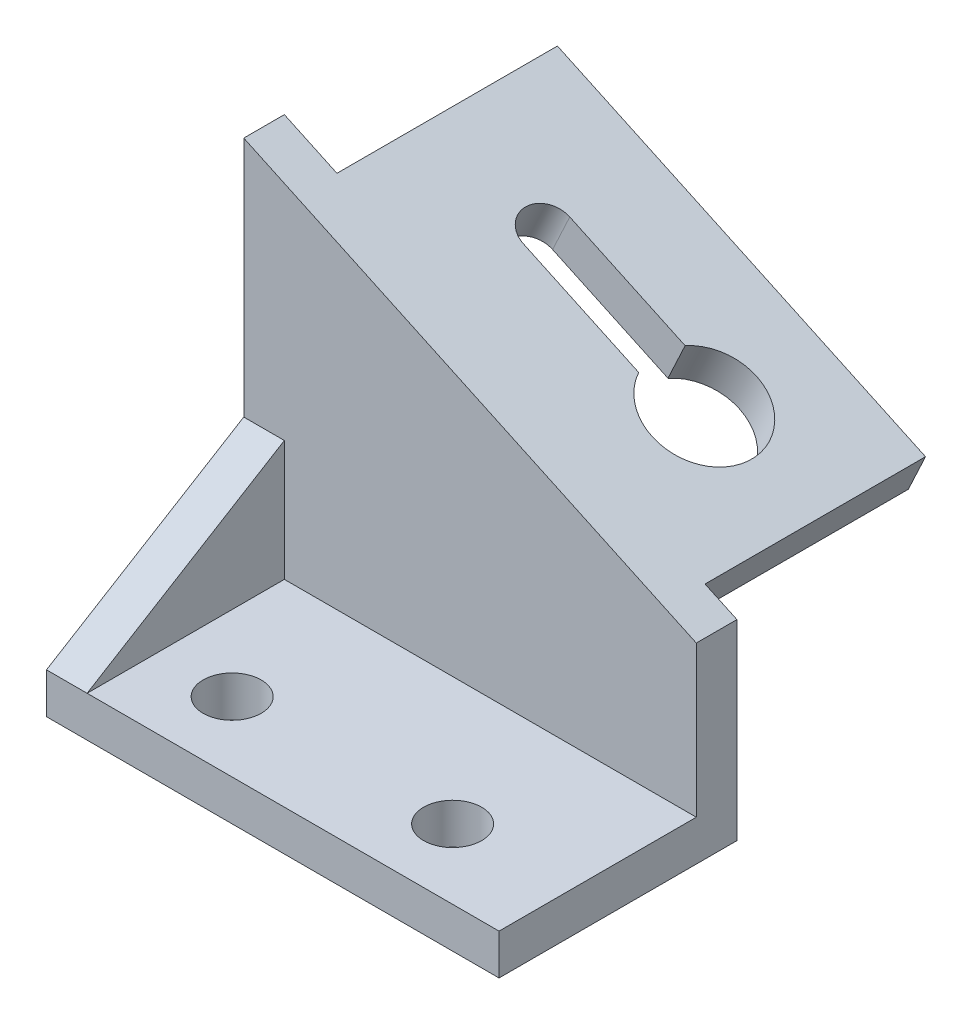
ISO-10303-21;
HEADER;
FILE_DESCRIPTION(('STEP AP214'),'2;1');
FILE_NAME('part.step','',(''),(''),'','','');
FILE_SCHEMA(('AUTOMOTIVE_DESIGN { 1 0 10303 214 1 1 1 1 }'));
ENDSEC;
DATA;
#1=APPLICATION_CONTEXT('core data for automotive mechanical design processes');
#2=APPLICATION_PROTOCOL_DEFINITION('international standard','automotive_design',2000,#1);
#3=PRODUCT_CONTEXT('',#1,'mechanical');
#4=PRODUCT('Part','Part','',(#3));
#5=PRODUCT_RELATED_PRODUCT_CATEGORY('part','',(#4));
#6=PRODUCT_DEFINITION_FORMATION('','',#4);
#7=PRODUCT_DEFINITION_CONTEXT('part definition',#1,'design');
#8=PRODUCT_DEFINITION('design','',#6,#7);
#9=PRODUCT_DEFINITION_SHAPE('','',#8);
#10=(LENGTH_UNIT() NAMED_UNIT(*) SI_UNIT(.MILLI.,.METRE.));
#11=(NAMED_UNIT(*) PLANE_ANGLE_UNIT() SI_UNIT($,.RADIAN.));
#12=(NAMED_UNIT(*) SI_UNIT($,.STERADIAN.) SOLID_ANGLE_UNIT());
#13=UNCERTAINTY_MEASURE_WITH_UNIT(LENGTH_MEASURE(1.E-05),#10,'distance_accuracy_value','');
#14=(GEOMETRIC_REPRESENTATION_CONTEXT(3) GLOBAL_UNCERTAINTY_ASSIGNED_CONTEXT((#13)) GLOBAL_UNIT_ASSIGNED_CONTEXT((#10,
#11,#12)) REPRESENTATION_CONTEXT('',''));
#15=CARTESIAN_POINT('',(0.,0.,0.));
#16=DIRECTION('',(0.,0.,1.));
#17=DIRECTION('',(1.,0.,0.));
#18=AXIS2_PLACEMENT_3D('',#15,#16,#17);
#19=CARTESIAN_POINT('',(-39.,7.,-20.5));
#20=DIRECTION('',(0.,0.,1.));
#21=DIRECTION('',(1.,0.,0.));
#22=AXIS2_PLACEMENT_3D('',#19,#20,#21);
#23=PLANE('',#22);
#24=DIRECTION('',(0.422618261740701,0.906307787036649,0.));
#25=VECTOR('',#24,1.);
#26=CARTESIAN_POINT('',(-32.8952499618184,58.8016602094265,-20.5));
#27=LINE('',#26,#25);
#28=CARTESIAN_POINT('',(-32.8952499618184,58.8016602094265,-20.5));
#29=VERTEX_POINT('',#28);
#30=CARTESIAN_POINT('',(-29.9369221296335,65.145814718683,-20.5));
#31=VERTEX_POINT('',#30);
#32=EDGE_CURVE('E202',#29,#31,#27,.T.);
#33=ORIENTED_EDGE('',*,*,#32,.F.);
#34=DIRECTION('',(0.906307787036649,-0.422618261740701,0.));
#35=VECTOR('',#34,1.);
#36=CARTESIAN_POINT('',(-32.8952499618184,58.8016602094265,-20.5));
#37=LINE('',#36,#35);
#38=CARTESIAN_POINT('',(30.5462951307471,29.2183818875774,-20.5));
#39=VERTEX_POINT('',#38);
#40=EDGE_CURVE('E193',#29,#39,#37,.T.);
#41=ORIENTED_EDGE('',*,*,#40,.T.);
#42=DIRECTION('',(0.422618261740701,0.906307787036649,0.));
#43=VECTOR('',#42,1.);
#44=CARTESIAN_POINT('',(30.5462951307471,29.2183818875774,-20.5));
#45=LINE('',#44,#43);
#46=CARTESIAN_POINT('',(33.504622962932,35.562536396834,-20.5));
#47=VERTEX_POINT('',#46);
#48=EDGE_CURVE('E216',#39,#47,#45,.T.);
#49=ORIENTED_EDGE('',*,*,#48,.T.);
#50=DIRECTION('',(0.906307787036649,-0.422618261740701,0.));
#51=VECTOR('',#50,1.);
#52=CARTESIAN_POINT('',(39.,33.,-20.5));
#53=LINE('',#52,#51);
#54=CARTESIAN_POINT('',(39.,33.,-20.5));
#55=VERTEX_POINT('',#54);
#56=EDGE_CURVE('E213',#47,#55,#53,.T.);
#57=ORIENTED_EDGE('',*,*,#56,.T.);
#58=DIRECTION('',(0.,-1.,0.));
#59=VECTOR('',#58,1.);
#60=CARTESIAN_POINT('',(39.,7.,-20.5));
#61=LINE('',#60,#59);
#62=CARTESIAN_POINT('',(39.,0.,-20.5));
#63=VERTEX_POINT('',#62);
#64=EDGE_CURVE('E50',#55,#63,#61,.T.);
#65=ORIENTED_EDGE('',*,*,#64,.T.);
#66=DIRECTION('',(-1.,0.,0.));
#67=VECTOR('',#66,1.);
#68=CARTESIAN_POINT('',(-39.,0.,-20.5));
#69=LINE('',#68,#67);
#70=CARTESIAN_POINT('',(-39.,0.,-20.5));
#71=VERTEX_POINT('',#70);
#72=EDGE_CURVE('E275',#63,#71,#69,.T.);
#73=ORIENTED_EDGE('',*,*,#72,.T.);
#74=DIRECTION('',(0.,-1.,0.));
#75=VECTOR('',#74,1.);
#76=CARTESIAN_POINT('',(-39.,7.,-20.5));
#77=LINE('',#76,#75);
#78=CARTESIAN_POINT('',(-39.,69.37199733609,-20.5));
#79=VERTEX_POINT('',#78);
#80=EDGE_CURVE('E282',#79,#71,#77,.T.);
#81=ORIENTED_EDGE('',*,*,#80,.F.);
#82=EDGE_CURVE('E224',#79,#31,#53,.T.);
#83=ORIENTED_EDGE('',*,*,#82,.T.);
#84=EDGE_LOOP('',(#33,#41,#49,#57,#65,#73,#81,#83));
#85=FACE_BOUND('',#84,.T.);
#86=ADVANCED_FACE('F39',(#85),#23,.F.);
#87=CARTESIAN_POINT('',(0.,7.,0.));
#88=DIRECTION('',(0.,1.,0.));
#89=DIRECTION('',(0.,0.,1.));
#90=AXIS2_PLACEMENT_3D('',#87,#88,#89);
#91=PLANE('',#90);
#92=CARTESIAN_POINT('',(-19.,7.,8.5));
#93=DIRECTION('',(0.,1.,0.));
#94=DIRECTION('',(0.,0.,1.));
#95=AXIS2_PLACEMENT_3D('',#92,#93,#94);
#96=CIRCLE('',#95,5.);
#97=CARTESIAN_POINT('',(-19.,7.,13.5));
#98=VERTEX_POINT('',#97);
#99=EDGE_CURVE('E254',#98,#98,#96,.T.);
#100=ORIENTED_EDGE('',*,*,#99,.F.);
#101=EDGE_LOOP('',(#100));
#102=FACE_BOUND('',#101,.T.);
#103=CARTESIAN_POINT('',(19.,7.,8.5));
#104=DIRECTION('',(0.,1.,0.));
#105=DIRECTION('',(0.,0.,1.));
#106=AXIS2_PLACEMENT_3D('',#103,#104,#105);
#107=CIRCLE('',#106,5.);
#108=CARTESIAN_POINT('',(19.,7.,13.5));
#109=VERTEX_POINT('',#108);
#110=EDGE_CURVE('E246',#109,#109,#107,.T.);
#111=ORIENTED_EDGE('',*,*,#110,.F.);
#112=EDGE_LOOP('',(#111));
#113=FACE_BOUND('',#112,.T.);
#114=DIRECTION('',(0.,0.,-1.));
#115=VECTOR('',#114,1.);
#116=CARTESIAN_POINT('',(39.,7.,-20.5));
#117=LINE('',#116,#115);
#118=CARTESIAN_POINT('',(39.,7.,20.5));
#119=VERTEX_POINT('',#118);
#120=CARTESIAN_POINT('',(39.,7.,-13.5));
#121=VERTEX_POINT('',#120);
#122=EDGE_CURVE('E261',#119,#121,#117,.T.);
#123=ORIENTED_EDGE('',*,*,#122,.T.);
#124=DIRECTION('',(-1.,0.,0.));
#125=VECTOR('',#124,1.);
#126=CARTESIAN_POINT('',(-39.,7.,-13.5));
#127=LINE('',#126,#125);
#128=CARTESIAN_POINT('',(-32.,7.,-13.5));
#129=VERTEX_POINT('',#128);
#130=EDGE_CURVE('E218',#121,#129,#127,.T.);
#131=ORIENTED_EDGE('',*,*,#130,.T.);
#132=DIRECTION('',(0.,0.,1.));
#133=VECTOR('',#132,1.);
#134=CARTESIAN_POINT('',(-32.,7.,-20.5));
#135=LINE('',#134,#133);
#136=CARTESIAN_POINT('',(-32.,7.,20.5));
#137=VERTEX_POINT('',#136);
#138=EDGE_CURVE('E243',#129,#137,#135,.T.);
#139=ORIENTED_EDGE('',*,*,#138,.T.);
#140=DIRECTION('',(1.,0.,0.));
#141=VECTOR('',#140,1.);
#142=CARTESIAN_POINT('',(-39.,7.,20.5));
#143=LINE('',#142,#141);
#144=EDGE_CURVE('E262',#137,#119,#143,.T.);
#145=ORIENTED_EDGE('',*,*,#144,.T.);
#146=EDGE_LOOP('',(#123,#131,#139,#145));
#147=FACE_BOUND('',#146,.T.);
#148=ADVANCED_FACE('F320',(#102,#113,#147),#91,.T.);
#149=CARTESIAN_POINT('',(0.,0.,0.));
#150=DIRECTION('',(0.,1.,0.));
#151=DIRECTION('',(0.,0.,1.));
#152=AXIS2_PLACEMENT_3D('',#149,#150,#151);
#153=PLANE('',#152);
#154=DIRECTION('',(0.,0.,-1.));
#155=VECTOR('',#154,1.);
#156=CARTESIAN_POINT('',(39.,0.,-20.5));
#157=LINE('',#156,#155);
#158=CARTESIAN_POINT('',(39.,0.,20.5));
#159=VERTEX_POINT('',#158);
#160=EDGE_CURVE('E256',#159,#63,#157,.T.);
#161=ORIENTED_EDGE('',*,*,#160,.F.);
#162=DIRECTION('',(1.,0.,0.));
#163=VECTOR('',#162,1.);
#164=CARTESIAN_POINT('',(-39.,0.,20.5));
#165=LINE('',#164,#163);
#166=CARTESIAN_POINT('',(-39.,0.,20.5));
#167=VERTEX_POINT('',#166);
#168=EDGE_CURVE('E264',#167,#159,#165,.T.);
#169=ORIENTED_EDGE('',*,*,#168,.F.);
#170=DIRECTION('',(0.,0.,1.));
#171=VECTOR('',#170,1.);
#172=CARTESIAN_POINT('',(-39.,0.,-20.5));
#173=LINE('',#172,#171);
#174=EDGE_CURVE('E274',#71,#167,#173,.T.);
#175=ORIENTED_EDGE('',*,*,#174,.F.);
#176=ORIENTED_EDGE('',*,*,#72,.F.);
#177=EDGE_LOOP('',(#161,#169,#175,#176));
#178=FACE_BOUND('',#177,.T.);
#179=CARTESIAN_POINT('',(-19.,0.,8.5));
#180=DIRECTION('',(0.,1.,0.));
#181=DIRECTION('',(0.,0.,1.));
#182=AXIS2_PLACEMENT_3D('',#179,#180,#181);
#183=CIRCLE('',#182,5.);
#184=CARTESIAN_POINT('',(-19.,0.,13.5));
#185=VERTEX_POINT('',#184);
#186=EDGE_CURVE('E252',#185,#185,#183,.T.);
#187=ORIENTED_EDGE('',*,*,#186,.T.);
#188=EDGE_LOOP('',(#187));
#189=FACE_BOUND('',#188,.T.);
#190=CARTESIAN_POINT('',(19.,0.,8.5));
#191=DIRECTION('',(0.,1.,0.));
#192=DIRECTION('',(0.,0.,1.));
#193=AXIS2_PLACEMENT_3D('',#190,#191,#192);
#194=CIRCLE('',#193,5.);
#195=CARTESIAN_POINT('',(19.,0.,13.5));
#196=VERTEX_POINT('',#195);
#197=EDGE_CURVE('E247',#196,#196,#194,.T.);
#198=ORIENTED_EDGE('',*,*,#197,.T.);
#199=EDGE_LOOP('',(#198));
#200=FACE_BOUND('',#199,.T.);
#201=ADVANCED_FACE('F298',(#178,#189,#200),#153,.F.);
#202=CARTESIAN_POINT('',(39.,7.,-20.5));
#203=DIRECTION('',(-1.,0.,0.));
#204=DIRECTION('',(0.,0.,1.));
#205=AXIS2_PLACEMENT_3D('',#202,#203,#204);
#206=PLANE('',#205);
#207=ORIENTED_EDGE('',*,*,#160,.T.);
#208=ORIENTED_EDGE('',*,*,#64,.F.);
#209=DIRECTION('',(0.,0.,-1.));
#210=VECTOR('',#209,1.);
#211=CARTESIAN_POINT('',(39.,33.,-13.5));
#212=LINE('',#211,#210);
#213=CARTESIAN_POINT('',(39.,33.,-13.5));
#214=VERTEX_POINT('',#213);
#215=EDGE_CURVE('E231',#214,#55,#212,.T.);
#216=ORIENTED_EDGE('',*,*,#215,.F.);
#217=DIRECTION('',(0.,-1.,0.));
#218=VECTOR('',#217,1.);
#219=CARTESIAN_POINT('',(39.,7.,-13.5));
#220=LINE('',#219,#218);
#221=EDGE_CURVE('E227',#214,#121,#220,.T.);
#222=ORIENTED_EDGE('',*,*,#221,.T.);
#223=ORIENTED_EDGE('',*,*,#122,.F.);
#224=DIRECTION('',(0.,-1.,0.));
#225=VECTOR('',#224,1.);
#226=CARTESIAN_POINT('',(39.,7.,20.5));
#227=LINE('',#226,#225);
#228=EDGE_CURVE('E267',#119,#159,#227,.T.);
#229=ORIENTED_EDGE('',*,*,#228,.T.);
#230=EDGE_LOOP('',(#207,#208,#216,#222,#223,#229));
#231=FACE_BOUND('',#230,.T.);
#232=ADVANCED_FACE('F41',(#231),#206,.F.);
#233=CARTESIAN_POINT('',(-39.,7.,-20.5));
#234=DIRECTION('',(1.,0.,0.));
#235=DIRECTION('',(0.,0.,-1.));
#236=AXIS2_PLACEMENT_3D('',#233,#234,#235);
#237=PLANE('',#236);
#238=ORIENTED_EDGE('',*,*,#80,.T.);
#239=ORIENTED_EDGE('',*,*,#174,.T.);
#240=DIRECTION('',(0.,-1.,0.));
#241=VECTOR('',#240,1.);
#242=CARTESIAN_POINT('',(-39.,7.,20.5));
#243=LINE('',#242,#241);
#244=CARTESIAN_POINT('',(-39.,7.,20.5));
#245=VERTEX_POINT('',#244);
#246=EDGE_CURVE('E278',#245,#167,#243,.T.);
#247=ORIENTED_EDGE('',*,*,#246,.F.);
#248=DIRECTION('',(0.,0.520607424264656,-0.853796175794036));
#249=VECTOR('',#248,1.);
#250=CARTESIAN_POINT('',(-39.,7.,20.5));
#251=LINE('',#250,#249);
#252=CARTESIAN_POINT('',(-39.,27.7317073170732,-13.5));
#253=VERTEX_POINT('',#252);
#254=EDGE_CURVE('E238',#245,#253,#251,.T.);
#255=ORIENTED_EDGE('',*,*,#254,.T.);
#256=DIRECTION('',(0.,1.,0.));
#257=VECTOR('',#256,1.);
#258=CARTESIAN_POINT('',(-39.,69.37199733609,-13.5));
#259=LINE('',#258,#257);
#260=CARTESIAN_POINT('',(-39.,69.37199733609,-13.5));
#261=VERTEX_POINT('',#260);
#262=EDGE_CURVE('E225',#253,#261,#259,.T.);
#263=ORIENTED_EDGE('',*,*,#262,.T.);
#264=DIRECTION('',(0.,0.,-1.));
#265=VECTOR('',#264,1.);
#266=CARTESIAN_POINT('',(-39.,69.37199733609,-13.5));
#267=LINE('',#266,#265);
#268=EDGE_CURVE('E232',#261,#79,#267,.T.);
#269=ORIENTED_EDGE('',*,*,#268,.T.);
#270=EDGE_LOOP('',(#238,#239,#247,#255,#263,#269));
#271=FACE_BOUND('',#270,.T.);
#272=ADVANCED_FACE('F296',(#271),#237,.F.);
#273=CARTESIAN_POINT('',(-39.,7.,20.5));
#274=DIRECTION('',(0.,0.,-1.));
#275=DIRECTION('',(-1.,0.,0.));
#276=AXIS2_PLACEMENT_3D('',#273,#274,#275);
#277=PLANE('',#276);
#278=ORIENTED_EDGE('',*,*,#168,.T.);
#279=ORIENTED_EDGE('',*,*,#228,.F.);
#280=ORIENTED_EDGE('',*,*,#144,.F.);
#281=EDGE_CURVE('E266',#245,#137,#143,.T.);
#282=ORIENTED_EDGE('',*,*,#281,.F.);
#283=ORIENTED_EDGE('',*,*,#246,.T.);
#284=EDGE_LOOP('',(#278,#279,#280,#282,#283));
#285=FACE_BOUND('',#284,.T.);
#286=ADVANCED_FACE('F305',(#285),#277,.F.);
#287=CARTESIAN_POINT('',(-19.,7.,8.5));
#288=DIRECTION('',(0.,-1.,0.));
#289=DIRECTION('',(0.,0.,-1.));
#290=AXIS2_PLACEMENT_3D('',#287,#288,#289);
#291=CYLINDRICAL_SURFACE('',#290,5.);
#292=ORIENTED_EDGE('',*,*,#99,.T.);
#293=EDGE_LOOP('',(#292));
#294=FACE_BOUND('',#293,.T.);
#295=ORIENTED_EDGE('',*,*,#186,.F.);
#296=EDGE_LOOP('',(#295));
#297=FACE_BOUND('',#296,.T.);
#298=ADVANCED_FACE('F344',(#294,#297),#291,.F.);
#299=CARTESIAN_POINT('',(19.,7.,8.5));
#300=DIRECTION('',(0.,-1.,0.));
#301=DIRECTION('',(0.,0.,-1.));
#302=AXIS2_PLACEMENT_3D('',#299,#300,#301);
#303=CYLINDRICAL_SURFACE('',#302,5.);
#304=ORIENTED_EDGE('',*,*,#110,.T.);
#305=EDGE_LOOP('',(#304));
#306=FACE_BOUND('',#305,.T.);
#307=ORIENTED_EDGE('',*,*,#197,.F.);
#308=EDGE_LOOP('',(#307));
#309=FACE_BOUND('',#308,.T.);
#310=ADVANCED_FACE('F328',(#306,#309),#303,.F.);
#311=CARTESIAN_POINT('',(-32.,7.,20.5));
#312=DIRECTION('',(0.,0.853796175794036,0.520607424264656));
#313=DIRECTION('',(0.,-0.520607424264656,0.853796175794036));
#314=AXIS2_PLACEMENT_3D('',#311,#312,#313);
#315=PLANE('',#314);
#316=DIRECTION('',(1.,0.,0.));
#317=VECTOR('',#316,1.);
#318=CARTESIAN_POINT('',(-32.,27.7317073170732,-13.5));
#319=LINE('',#318,#317);
#320=CARTESIAN_POINT('',(-32.,27.7317073170732,-13.5));
#321=VERTEX_POINT('',#320);
#322=EDGE_CURVE('E64',#253,#321,#319,.T.);
#323=ORIENTED_EDGE('',*,*,#322,.F.);
#324=ORIENTED_EDGE('',*,*,#254,.F.);
#325=ORIENTED_EDGE('',*,*,#281,.T.);
#326=DIRECTION('',(0.,0.520607424264656,-0.853796175794036));
#327=VECTOR('',#326,1.);
#328=CARTESIAN_POINT('',(-32.,7.,20.5));
#329=LINE('',#328,#327);
#330=EDGE_CURVE('E242',#137,#321,#329,.T.);
#331=ORIENTED_EDGE('',*,*,#330,.T.);
#332=EDGE_LOOP('',(#323,#324,#325,#331));
#333=FACE_BOUND('',#332,.T.);
#334=ADVANCED_FACE('F308',(#333),#315,.T.);
#335=CARTESIAN_POINT('',(-32.,0.,0.));
#336=DIRECTION('',(-1.,0.,0.));
#337=DIRECTION('',(0.,0.,1.));
#338=AXIS2_PLACEMENT_3D('',#335,#336,#337);
#339=PLANE('',#338);
#340=ORIENTED_EDGE('',*,*,#138,.F.);
#341=DIRECTION('',(0.,1.,0.));
#342=VECTOR('',#341,1.);
#343=CARTESIAN_POINT('',(-32.,0.,-13.5));
#344=LINE('',#343,#342);
#345=EDGE_CURVE('E11',#129,#321,#344,.T.);
#346=ORIENTED_EDGE('',*,*,#345,.T.);
#347=ORIENTED_EDGE('',*,*,#330,.F.);
#348=EDGE_LOOP('',(#340,#346,#347));
#349=FACE_BOUND('',#348,.T.);
#350=ADVANCED_FACE('F319',(#349),#339,.F.);
#351=CARTESIAN_POINT('',(39.,33.,-13.5));
#352=DIRECTION('',(0.422618261740701,0.906307787036649,0.));
#353=DIRECTION('',(-0.906307787036649,0.422618261740701,0.));
#354=AXIS2_PLACEMENT_3D('',#351,#352,#353);
#355=PLANE('',#354);
#356=ORIENTED_EDGE('',*,*,#82,.F.);
#357=ORIENTED_EDGE('',*,*,#268,.F.);
#358=DIRECTION('',(0.906307787036649,-0.422618261740701,0.));
#359=VECTOR('',#358,1.);
#360=CARTESIAN_POINT('',(39.,33.,-13.5));
#361=LINE('',#360,#359);
#362=EDGE_CURVE('E223',#261,#214,#361,.T.);
#363=ORIENTED_EDGE('',*,*,#362,.T.);
#364=ORIENTED_EDGE('',*,*,#215,.T.);
#365=ORIENTED_EDGE('',*,*,#56,.F.);
#366=DIRECTION('',(0.,0.,-1.));
#367=VECTOR('',#366,1.);
#368=CARTESIAN_POINT('',(33.504622962932,35.562536396834,-20.5));
#369=LINE('',#368,#367);
#370=CARTESIAN_POINT('',(33.504622962932,35.562536396834,-58.5));
#371=VERTEX_POINT('',#370);
#372=EDGE_CURVE('E53',#47,#371,#369,.T.);
#373=ORIENTED_EDGE('',*,*,#372,.T.);
#374=DIRECTION('',(-0.906307787036649,0.422618261740701,0.));
#375=VECTOR('',#374,1.);
#376=CARTESIAN_POINT('',(-29.9369221296335,65.145814718683,-58.5));
#377=LINE('',#376,#375);
#378=CARTESIAN_POINT('',(-29.9369221296335,65.145814718683,-58.5));
#379=VERTEX_POINT('',#378);
#380=EDGE_CURVE('E198',#371,#379,#377,.T.);
#381=ORIENTED_EDGE('',*,*,#380,.T.);
#382=DIRECTION('',(0.,0.,1.));
#383=VECTOR('',#382,1.);
#384=CARTESIAN_POINT('',(-29.9369221296335,65.145814718683,-20.5));
#385=LINE('',#384,#383);
#386=EDGE_CURVE('E187',#379,#31,#385,.T.);
#387=ORIENTED_EDGE('',*,*,#386,.T.);
#388=EDGE_LOOP('',(#356,#357,#363,#364,#365,#373,#381,#387));
#389=FACE_BOUND('',#388,.T.);
#390=DIRECTION('',(0.906307787036649,-0.422618261740701,0.));
#391=VECTOR('',#390,1.);
#392=CARTESIAN_POINT('',(-11.8107663889005,56.693449483869,-34.5));
#393=LINE('',#392,#391);
#394=CARTESIAN_POINT('',(-11.8107663889005,56.693449483869,-34.5));
#395=VERTEX_POINT('',#394);
#396=CARTESIAN_POINT('',(8.07158024381943,47.4221589869394,-34.5));
#397=VERTEX_POINT('',#396);
#398=EDGE_CURVE('E185',#395,#397,#393,.T.);
#399=ORIENTED_EDGE('',*,*,#398,.F.);
#400=CARTESIAN_POINT('',(-11.8107663889005,56.693449483869,-38.5));
#401=DIRECTION('',(0.422618261740701,0.906307787036649,0.));
#402=DIRECTION('',(-0.906307787036649,0.422618261740701,0.));
#403=AXIS2_PLACEMENT_3D('',#400,#401,#402);
#404=CIRCLE('',#403,4.);
#405=CARTESIAN_POINT('',(-11.8107663889005,56.693449483869,-42.5));
#406=VERTEX_POINT('',#405);
#407=EDGE_CURVE('E154',#406,#395,#404,.T.);
#408=ORIENTED_EDGE('',*,*,#407,.F.);
#409=DIRECTION('',(-0.906307787036649,0.422618261740701,0.));
#410=VECTOR('',#409,1.);
#411=CARTESIAN_POINT('',(-11.8107663889005,56.693449483869,-42.5));
#412=LINE('',#411,#410);
#413=CARTESIAN_POINT('',(8.07158024381943,47.4221589869394,-42.5));
#414=VERTEX_POINT('',#413);
#415=EDGE_CURVE('E172',#414,#406,#412,.T.);
#416=ORIENTED_EDGE('',*,*,#415,.F.);
#417=CARTESIAN_POINT('',(15.378467222199,44.014901631648,-38.5));
#418=DIRECTION('',(0.422618261740701,0.906307787036649,0.));
#419=DIRECTION('',(-0.906307787036649,0.422618261740701,0.));
#420=AXIS2_PLACEMENT_3D('',#417,#418,#419);
#421=CIRCLE('',#420,9.);
#422=EDGE_CURVE('E177',#397,#414,#421,.T.);
#423=ORIENTED_EDGE('',*,*,#422,.F.);
#424=EDGE_LOOP('',(#399,#408,#416,#423));
#425=FACE_BOUND('',#424,.T.);
#426=ADVANCED_FACE('F315',(#389,#425),#355,.T.);
#427=CARTESIAN_POINT('',(0.,0.,-13.5));
#428=DIRECTION('',(0.,0.,1.));
#429=DIRECTION('',(1.,0.,0.));
#430=AXIS2_PLACEMENT_3D('',#427,#428,#429);
#431=PLANE('',#430);
#432=ORIENTED_EDGE('',*,*,#262,.F.);
#433=ORIENTED_EDGE('',*,*,#322,.T.);
#434=ORIENTED_EDGE('',*,*,#345,.F.);
#435=ORIENTED_EDGE('',*,*,#130,.F.);
#436=ORIENTED_EDGE('',*,*,#221,.F.);
#437=ORIENTED_EDGE('',*,*,#362,.F.);
#438=EDGE_LOOP('',(#432,#433,#434,#435,#436,#437));
#439=FACE_BOUND('',#438,.T.);
#440=ADVANCED_FACE('F312',(#439),#431,.T.);
#441=CARTESIAN_POINT('',(-32.8952499618184,58.8016602094265,-20.5));
#442=DIRECTION('',(-0.906307787036649,0.422618261740701,0.));
#443=DIRECTION('',(-0.422618261740701,-0.906307787036649,0.));
#444=AXIS2_PLACEMENT_3D('',#441,#442,#443);
#445=PLANE('',#444);
#446=ORIENTED_EDGE('',*,*,#386,.F.);
#447=DIRECTION('',(0.422618261740701,0.906307787036649,0.));
#448=VECTOR('',#447,1.);
#449=CARTESIAN_POINT('',(-32.8952499618184,58.8016602094265,-58.5));
#450=LINE('',#449,#448);
#451=CARTESIAN_POINT('',(-32.8952499618184,58.8016602094265,-58.5));
#452=VERTEX_POINT('',#451);
#453=EDGE_CURVE('E211',#452,#379,#450,.T.);
#454=ORIENTED_EDGE('',*,*,#453,.F.);
#455=DIRECTION('',(0.,0.,1.));
#456=VECTOR('',#455,1.);
#457=CARTESIAN_POINT('',(-32.8952499618184,58.8016602094265,-20.5));
#458=LINE('',#457,#456);
#459=EDGE_CURVE('E194',#452,#29,#458,.T.);
#460=ORIENTED_EDGE('',*,*,#459,.T.);
#461=ORIENTED_EDGE('',*,*,#32,.T.);
#462=EDGE_LOOP('',(#446,#454,#460,#461));
#463=FACE_BOUND('',#462,.T.);
#464=ADVANCED_FACE('F408',(#463),#445,.T.);
#465=CARTESIAN_POINT('',(-32.8952499618184,58.8016602094265,-58.5));
#466=DIRECTION('',(0.,0.,-1.));
#467=DIRECTION('',(-1.,0.,0.));
#468=AXIS2_PLACEMENT_3D('',#465,#466,#467);
#469=PLANE('',#468);
#470=ORIENTED_EDGE('',*,*,#380,.F.);
#471=DIRECTION('',(0.422618261740701,0.906307787036649,0.));
#472=VECTOR('',#471,1.);
#473=CARTESIAN_POINT('',(30.5462951307471,29.2183818875774,-58.5));
#474=LINE('',#473,#472);
#475=CARTESIAN_POINT('',(30.5462951307471,29.2183818875774,-58.5));
#476=VERTEX_POINT('',#475);
#477=EDGE_CURVE('E212',#476,#371,#474,.T.);
#478=ORIENTED_EDGE('',*,*,#477,.F.);
#479=DIRECTION('',(-0.906307787036649,0.422618261740701,0.));
#480=VECTOR('',#479,1.);
#481=CARTESIAN_POINT('',(-32.8952499618184,58.8016602094265,-58.5));
#482=LINE('',#481,#480);
#483=EDGE_CURVE('E205',#476,#452,#482,.T.);
#484=ORIENTED_EDGE('',*,*,#483,.T.);
#485=ORIENTED_EDGE('',*,*,#453,.T.);
#486=EDGE_LOOP('',(#470,#478,#484,#485));
#487=FACE_BOUND('',#486,.T.);
#488=ADVANCED_FACE('F423',(#487),#469,.T.);
#489=CARTESIAN_POINT('',(30.5462951307471,29.2183818875774,-20.5));
#490=DIRECTION('',(0.906307787036649,-0.422618261740701,0.));
#491=DIRECTION('',(0.422618261740701,0.906307787036649,0.));
#492=AXIS2_PLACEMENT_3D('',#489,#490,#491);
#493=PLANE('',#492);
#494=ORIENTED_EDGE('',*,*,#372,.F.);
#495=ORIENTED_EDGE('',*,*,#48,.F.);
#496=DIRECTION('',(0.,0.,-1.));
#497=VECTOR('',#496,1.);
#498=CARTESIAN_POINT('',(30.5462951307471,29.2183818875774,-20.5));
#499=LINE('',#498,#497);
#500=EDGE_CURVE('E200',#39,#476,#499,.T.);
#501=ORIENTED_EDGE('',*,*,#500,.T.);
#502=ORIENTED_EDGE('',*,*,#477,.T.);
#503=EDGE_LOOP('',(#494,#495,#501,#502));
#504=FACE_BOUND('',#503,.T.);
#505=ADVANCED_FACE('F429',(#504),#493,.T.);
#506=CARTESIAN_POINT('',(16.6470470903908,35.6997076913915,0.));
#507=DIRECTION('',(-0.422618261740701,-0.906307787036649,0.));
#508=DIRECTION('',(0.906307787036649,-0.422618261740701,0.));
#509=AXIS2_PLACEMENT_3D('',#506,#507,#508);
#510=PLANE('',#509);
#511=CARTESIAN_POINT('',(-14.7690942210854,50.3492949746125,-38.5));
#512=DIRECTION('',(0.422618261740701,0.906307787036649,0.));
#513=DIRECTION('',(-0.906307787036649,0.422618261740701,0.));
#514=AXIS2_PLACEMENT_3D('',#511,#512,#513);
#515=CIRCLE('',#514,4.);
#516=CARTESIAN_POINT('',(-14.7690942210854,50.3492949746125,-42.5));
#517=VERTEX_POINT('',#516);
#518=CARTESIAN_POINT('',(-14.7690942210854,50.3492949746125,-34.5));
#519=VERTEX_POINT('',#518);
#520=EDGE_CURVE('E155',#517,#519,#515,.T.);
#521=ORIENTED_EDGE('',*,*,#520,.T.);
#522=DIRECTION('',(0.906307787036649,-0.422618261740701,0.));
#523=VECTOR('',#522,1.);
#524=CARTESIAN_POINT('',(-14.7690942210854,50.3492949746125,-34.5));
#525=LINE('',#524,#523);
#526=CARTESIAN_POINT('',(5.11325241163458,41.0780044776829,-34.5));
#527=VERTEX_POINT('',#526);
#528=EDGE_CURVE('E163',#519,#527,#525,.T.);
#529=ORIENTED_EDGE('',*,*,#528,.T.);
#530=CARTESIAN_POINT('',(12.4201393900141,37.6707471223914,-38.5));
#531=DIRECTION('',(0.422618261740701,0.906307787036649,0.));
#532=DIRECTION('',(-0.906307787036649,0.422618261740701,0.));
#533=AXIS2_PLACEMENT_3D('',#530,#531,#532);
#534=CIRCLE('',#533,9.);
#535=CARTESIAN_POINT('',(5.11325241163452,41.0780044776829,-42.5));
#536=VERTEX_POINT('',#535);
#537=EDGE_CURVE('E169',#527,#536,#534,.T.);
#538=ORIENTED_EDGE('',*,*,#537,.T.);
#539=DIRECTION('',(-0.906307787036649,0.422618261740701,0.));
#540=VECTOR('',#539,1.);
#541=CARTESIAN_POINT('',(-14.7690942210854,50.3492949746125,-42.5));
#542=LINE('',#541,#540);
#543=EDGE_CURVE('E159',#536,#517,#542,.T.);
#544=ORIENTED_EDGE('',*,*,#543,.T.);
#545=EDGE_LOOP('',(#521,#529,#538,#544));
#546=FACE_BOUND('',#545,.T.);
#547=ORIENTED_EDGE('',*,*,#459,.F.);
#548=ORIENTED_EDGE('',*,*,#483,.F.);
#549=ORIENTED_EDGE('',*,*,#500,.F.);
#550=ORIENTED_EDGE('',*,*,#40,.F.);
#551=EDGE_LOOP('',(#547,#548,#549,#550));
#552=FACE_BOUND('',#551,.T.);
#553=ADVANCED_FACE('F168',(#546,#552),#510,.T.);
#554=CARTESIAN_POINT('',(-14.7690942210854,50.3492949746125,-38.5));
#555=DIRECTION('',(0.422618261740701,0.906307787036649,0.));
#556=DIRECTION('',(-0.906307787036649,0.422618261740701,0.));
#557=AXIS2_PLACEMENT_3D('',#554,#555,#556);
#558=CYLINDRICAL_SURFACE('',#557,4.);
#559=ORIENTED_EDGE('',*,*,#407,.T.);
#560=DIRECTION('',(0.422618261740701,0.906307787036649,0.));
#561=VECTOR('',#560,1.);
#562=CARTESIAN_POINT('',(-14.7690942210854,50.3492949746125,-34.5));
#563=LINE('',#562,#561);
#564=EDGE_CURVE('E146',#519,#395,#563,.T.);
#565=ORIENTED_EDGE('',*,*,#564,.F.);
#566=ORIENTED_EDGE('',*,*,#520,.F.);
#567=DIRECTION('',(0.422618261740701,0.906307787036649,0.));
#568=VECTOR('',#567,1.);
#569=CARTESIAN_POINT('',(-14.7690942210854,50.3492949746125,-42.5));
#570=LINE('',#569,#568);
#571=EDGE_CURVE('E188',#517,#406,#570,.T.);
#572=ORIENTED_EDGE('',*,*,#571,.T.);
#573=EDGE_LOOP('',(#559,#565,#566,#572));
#574=FACE_BOUND('',#573,.T.);
#575=ADVANCED_FACE('F147',(#574),#558,.F.);
#576=CARTESIAN_POINT('',(-14.7690942210854,50.3492949746125,-42.5));
#577=DIRECTION('',(0.,0.,-1.));
#578=DIRECTION('',(-1.,0.,0.));
#579=AXIS2_PLACEMENT_3D('',#576,#577,#578);
#580=PLANE('',#579);
#581=ORIENTED_EDGE('',*,*,#415,.T.);
#582=ORIENTED_EDGE('',*,*,#571,.F.);
#583=ORIENTED_EDGE('',*,*,#543,.F.);
#584=DIRECTION('',(0.422618261740701,0.906307787036649,0.));
#585=VECTOR('',#584,1.);
#586=CARTESIAN_POINT('',(5.11325241163452,41.0780044776829,-42.5));
#587=LINE('',#586,#585);
#588=EDGE_CURVE('E190',#536,#414,#587,.T.);
#589=ORIENTED_EDGE('',*,*,#588,.T.);
#590=EDGE_LOOP('',(#581,#582,#583,#589));
#591=FACE_BOUND('',#590,.T.);
#592=ADVANCED_FACE('F455',(#591),#580,.F.);
#593=CARTESIAN_POINT('',(12.4201393900141,37.6707471223914,-38.5));
#594=DIRECTION('',(0.422618261740701,0.906307787036649,0.));
#595=DIRECTION('',(-0.906307787036649,0.422618261740701,0.));
#596=AXIS2_PLACEMENT_3D('',#593,#594,#595);
#597=CYLINDRICAL_SURFACE('',#596,9.);
#598=ORIENTED_EDGE('',*,*,#422,.T.);
#599=ORIENTED_EDGE('',*,*,#588,.F.);
#600=ORIENTED_EDGE('',*,*,#537,.F.);
#601=DIRECTION('',(0.422618261740701,0.906307787036649,0.));
#602=VECTOR('',#601,1.);
#603=CARTESIAN_POINT('',(5.11325241163452,41.0780044776829,-34.5));
#604=LINE('',#603,#602);
#605=EDGE_CURVE('E157',#527,#397,#604,.T.);
#606=ORIENTED_EDGE('',*,*,#605,.T.);
#607=EDGE_LOOP('',(#598,#599,#600,#606));
#608=FACE_BOUND('',#607,.T.);
#609=ADVANCED_FACE('F463',(#608),#597,.F.);
#610=CARTESIAN_POINT('',(-14.7690942210854,50.3492949746125,-34.5));
#611=DIRECTION('',(0.,0.,1.));
#612=DIRECTION('',(1.,0.,0.));
#613=AXIS2_PLACEMENT_3D('',#610,#611,#612);
#614=PLANE('',#613);
#615=ORIENTED_EDGE('',*,*,#398,.T.);
#616=ORIENTED_EDGE('',*,*,#605,.F.);
#617=ORIENTED_EDGE('',*,*,#528,.F.);
#618=ORIENTED_EDGE('',*,*,#564,.T.);
#619=EDGE_LOOP('',(#615,#616,#617,#618));
#620=FACE_BOUND('',#619,.T.);
#621=ADVANCED_FACE('F164',(#620),#614,.F.);
#622=CLOSED_SHELL('',(#86,#148,#201,#232,#272,#286,#298,#310,#334,#350,#426,#440,#464,#488,#505,
#553,#575,#592,#609,#621));
#623=MANIFOLD_SOLID_BREP('B2',#622);
#624=ADVANCED_BREP_SHAPE_REPRESENTATION('',(#18,#623),#14);
#625=SHAPE_DEFINITION_REPRESENTATION(#9,#624);
ENDSEC;
END-ISO-10303-21;
